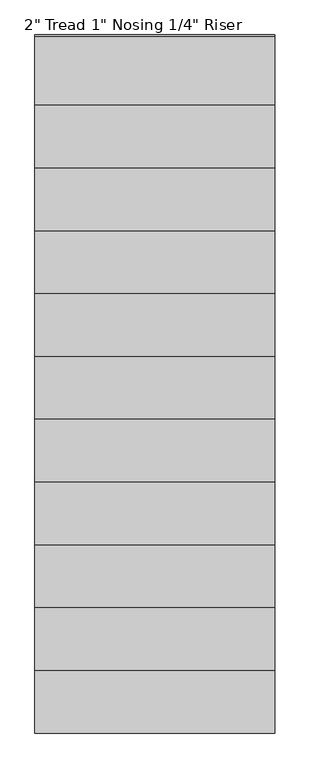
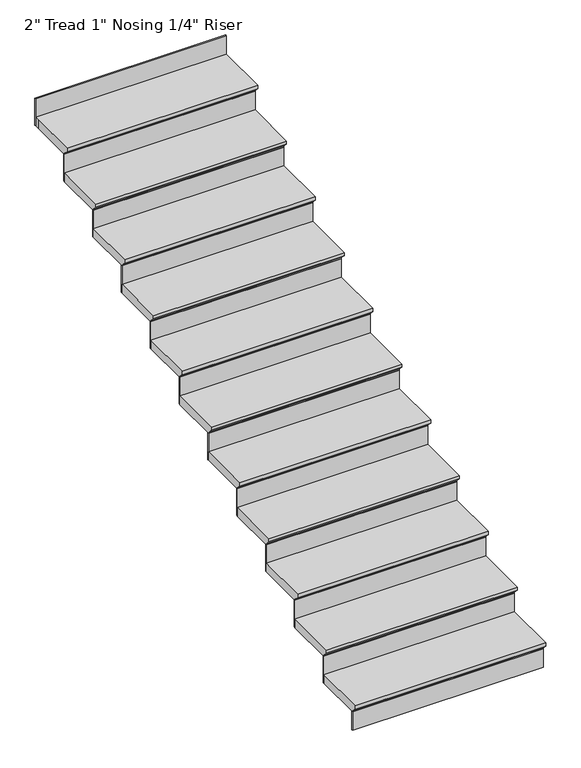
"""IFC4 building model written with IfcOpenShell, lengths in millimetres: stair flight geometry."""

from ifc_helpers import new_model, si_unit, origin, place, context, project, spatial, faceted_brep, source, transform, mapped, element, save


def stair_flight_4c38af94(model_context):
    return source(origin(), model_context, "Body", "Brep", [
        faceted_brep([(-5186.1338869, 1781.9468856, 141.3710526), (-5186.1338869, 1781.9468856, 160.4210526), (-6252.9338869, 1781.9468856, 160.4210526), (-6252.9338869, 1781.9468856, 141.3710526), (-5186.1338869, 1807.3468856, 115.9710526), (-6252.9338869, 1807.3468856, 115.9710526), (-5186.1338869, 2086.7468856, 160.4210526), (-6252.9338869, 2086.7468856, 160.4210526), (-6252.9338869, 1807.3468856, 109.6210526), (-6252.9338869, 2086.7468856, 109.6210526), (-5186.1338869, 2086.7468856, 109.6210526), (-5186.1338869, 1807.3468856, 109.6210526)], [[[0, 1, 2, 3]], [[4, 0, 3, 5]], [[2, 1, 6, 7]], [[8, 9, 10, 11]], [[2, 7, 9, 8, 5, 3]], [[8, 11, 4, 5]], [[6, 1, 0, 4, 11, 10]], [[7, 6, 10, 9]]]),
        faceted_brep([(-5186.1338869, 1807.3468856, 109.6210526), (-5186.1338869, 1807.3468856, 0.0), (-5186.1338869, 1813.6968856, 0.0), (-5186.1338869, 1813.6968856, 109.6210526), (-6252.9338869, 1807.3468856, 109.6210526), (-6252.9338869, 1813.6968856, 109.6210526), (-6252.9338869, 1813.6968856, 0.0), (-6252.9338869, 1807.3468856, 0.0)], [[[0, 1, 2, 3]], [[4, 5, 6, 7]], [[1, 0, 4, 7]], [[2, 1, 7, 6]], [[3, 2, 6, 5]], [[0, 3, 5, 4]]]),
        faceted_brep([(-5186.1338869, 2086.7468856, 270.0421053), (-5186.1338869, 2086.7468856, 109.6210526), (-5186.1338869, 2093.0968856, 109.6210526), (-5186.1338869, 2093.0968856, 270.0421053), (-6252.9338869, 2086.7468856, 270.0421053), (-6252.9338869, 2093.0968856, 270.0421053), (-6252.9338869, 2093.0968856, 109.6210526), (-6252.9338869, 2086.7468856, 109.6210526)], [[[0, 1, 2, 3]], [[4, 5, 6, 7]], [[1, 0, 4, 7]], [[2, 1, 7, 6]], [[3, 2, 6, 5]], [[0, 3, 5, 4]]]),
        faceted_brep([(-6252.9338869, 2061.3468856, 320.8421053), (-5186.1338869, 2061.3468856, 320.8421053), (-5186.1338869, 2366.1468856, 320.8421053), (-6252.9338869, 2366.1468856, 320.8421053), (-6252.9338869, 2086.7468856, 270.0421053), (-6252.9338869, 2366.1468856, 270.0421053), (-5186.1338869, 2366.1468856, 270.0421053), (-5186.1338869, 2086.7468856, 270.0421053), (-6252.9338869, 2086.7468856, 276.3921053), (-6252.9338869, 2061.3468856, 301.7921053), (-5186.1338869, 2086.7468856, 276.3921053), (-5186.1338869, 2061.3468856, 301.7921053)], [[[0, 1, 2, 3]], [[4, 5, 6, 7]], [[0, 3, 5, 4, 8, 9]], [[4, 7, 10, 8]], [[2, 1, 11, 10, 7, 6]], [[3, 2, 6, 5]], [[11, 1, 0, 9]], [[10, 11, 9, 8]]]),
        faceted_brep([(-5186.1338869, 2366.1468856, 430.4631579), (-5186.1338869, 2366.1468856, 270.0421053), (-5186.1338869, 2372.4968856, 270.0421053), (-5186.1338869, 2372.4968856, 430.4631579), (-6252.9338869, 2366.1468856, 430.4631579), (-6252.9338869, 2372.4968856, 430.4631579), (-6252.9338869, 2372.4968856, 270.0421053), (-6252.9338869, 2366.1468856, 270.0421053)], [[[0, 1, 2, 3]], [[4, 5, 6, 7]], [[1, 0, 4, 7]], [[2, 1, 7, 6]], [[3, 2, 6, 5]], [[0, 3, 5, 4]]]),
        faceted_brep([(-6252.9338869, 2340.7468856, 481.2631579), (-5186.1338869, 2340.7468856, 481.2631579), (-5186.1338869, 2645.5468856, 481.2631579), (-6252.9338869, 2645.5468856, 481.2631579), (-6252.9338869, 2366.1468856, 430.4631579), (-6252.9338869, 2645.5468856, 430.4631579), (-5186.1338869, 2645.5468856, 430.4631579), (-5186.1338869, 2366.1468856, 430.4631579), (-6252.9338869, 2366.1468856, 436.8131579), (-6252.9338869, 2340.7468856, 462.2131579), (-5186.1338869, 2366.1468856, 436.8131579), (-5186.1338869, 2340.7468856, 462.2131579)], [[[0, 1, 2, 3]], [[4, 5, 6, 7]], [[0, 3, 5, 4, 8, 9]], [[4, 7, 10, 8]], [[2, 1, 11, 10, 7, 6]], [[3, 2, 6, 5]], [[11, 1, 0, 9]], [[10, 11, 9, 8]]]),
        faceted_brep([(-5186.1338869, 2645.5468856, 590.8842105), (-5186.1338869, 2645.5468856, 430.4631579), (-5186.1338869, 2651.8968856, 430.4631579), (-5186.1338869, 2651.8968856, 590.8842105), (-6252.9338869, 2645.5468856, 590.8842105), (-6252.9338869, 2651.8968856, 590.8842105), (-6252.9338869, 2651.8968856, 430.4631579), (-6252.9338869, 2645.5468856, 430.4631579)], [[[0, 1, 2, 3]], [[4, 5, 6, 7]], [[1, 0, 4, 7]], [[2, 1, 7, 6]], [[3, 2, 6, 5]], [[0, 3, 5, 4]]]),
        faceted_brep([(-6252.9338869, 2620.1468856, 641.6842105), (-5186.1338869, 2620.1468856, 641.6842105), (-5186.1338869, 2924.9468856, 641.6842105), (-6252.9338869, 2924.9468856, 641.6842105), (-6252.9338869, 2645.5468856, 590.8842105), (-6252.9338869, 2924.9468856, 590.8842105), (-5186.1338869, 2924.9468856, 590.8842105), (-5186.1338869, 2645.5468856, 590.8842105), (-6252.9338869, 2645.5468856, 597.2342105), (-6252.9338869, 2620.1468856, 622.6342105), (-5186.1338869, 2645.5468856, 597.2342105), (-5186.1338869, 2620.1468856, 622.6342105)], [[[0, 1, 2, 3]], [[4, 5, 6, 7]], [[0, 3, 5, 4, 8, 9]], [[4, 7, 10, 8]], [[2, 1, 11, 10, 7, 6]], [[3, 2, 6, 5]], [[11, 1, 0, 9]], [[10, 11, 9, 8]]]),
        faceted_brep([(-5186.1338869, 2924.9468856, 751.3052632), (-5186.1338869, 2924.9468856, 590.8842105), (-5186.1338869, 2931.2968856, 590.8842105), (-5186.1338869, 2931.2968856, 751.3052632), (-6252.9338869, 2924.9468856, 751.3052632), (-6252.9338869, 2931.2968856, 751.3052632), (-6252.9338869, 2931.2968856, 590.8842105), (-6252.9338869, 2924.9468856, 590.8842105)], [[[0, 1, 2, 3]], [[4, 5, 6, 7]], [[1, 0, 4, 7]], [[2, 1, 7, 6]], [[3, 2, 6, 5]], [[0, 3, 5, 4]]]),
        faceted_brep([(-6252.9338869, 2899.5468856, 802.1052632), (-5186.1338869, 2899.5468856, 802.1052632), (-5186.1338869, 3204.3468856, 802.1052632), (-6252.9338869, 3204.3468856, 802.1052632), (-6252.9338869, 2924.9468856, 751.3052632), (-6252.9338869, 3204.3468856, 751.3052632), (-5186.1338869, 3204.3468856, 751.3052632), (-5186.1338869, 2924.9468856, 751.3052632), (-6252.9338869, 2924.9468856, 757.6552632), (-6252.9338869, 2899.5468856, 783.0552632), (-5186.1338869, 2924.9468856, 757.6552632), (-5186.1338869, 2899.5468856, 783.0552632)], [[[0, 1, 2, 3]], [[4, 5, 6, 7]], [[0, 3, 5, 4, 8, 9]], [[4, 7, 10, 8]], [[2, 1, 11, 10, 7, 6]], [[3, 2, 6, 5]], [[11, 1, 0, 9]], [[10, 11, 9, 8]]]),
        faceted_brep([(-5186.1338869, 3204.3468856, 911.7263158), (-5186.1338869, 3204.3468856, 751.3052632), (-5186.1338869, 3210.6968856, 751.3052632), (-5186.1338869, 3210.6968856, 911.7263158), (-6252.9338869, 3204.3468856, 911.7263158), (-6252.9338869, 3210.6968856, 911.7263158), (-6252.9338869, 3210.6968856, 751.3052632), (-6252.9338869, 3204.3468856, 751.3052632)], [[[0, 1, 2, 3]], [[4, 5, 6, 7]], [[1, 0, 4, 7]], [[2, 1, 7, 6]], [[3, 2, 6, 5]], [[0, 3, 5, 4]]]),
        faceted_brep([(-6252.9338869, 3178.9468856, 962.5263158), (-5186.1338869, 3178.9468856, 962.5263158), (-5186.1338869, 3483.7468856, 962.5263158), (-6252.9338869, 3483.7468856, 962.5263158), (-6252.9338869, 3204.3468856, 911.7263158), (-6252.9338869, 3483.7468856, 911.7263158), (-5186.1338869, 3483.7468856, 911.7263158), (-5186.1338869, 3204.3468856, 911.7263158), (-6252.9338869, 3204.3468856, 918.0763158), (-6252.9338869, 3178.9468856, 943.4763158), (-5186.1338869, 3204.3468856, 918.0763158), (-5186.1338869, 3178.9468856, 943.4763158)], [[[0, 1, 2, 3]], [[4, 5, 6, 7]], [[0, 3, 5, 4, 8, 9]], [[4, 7, 10, 8]], [[2, 1, 11, 10, 7, 6]], [[3, 2, 6, 5]], [[11, 1, 0, 9]], [[10, 11, 9, 8]]]),
        faceted_brep([(-5186.1338869, 3483.7468856, 1072.1473684), (-5186.1338869, 3483.7468856, 911.7263158), (-5186.1338869, 3490.0968856, 911.7263158), (-5186.1338869, 3490.0968856, 1072.1473684), (-6252.9338869, 3483.7468856, 1072.1473684), (-6252.9338869, 3490.0968856, 1072.1473684), (-6252.9338869, 3490.0968856, 911.7263158), (-6252.9338869, 3483.7468856, 911.7263158)], [[[0, 1, 2, 3]], [[4, 5, 6, 7]], [[1, 0, 4, 7]], [[2, 1, 7, 6]], [[3, 2, 6, 5]], [[0, 3, 5, 4]]]),
        faceted_brep([(-6252.9338869, 3458.3468856, 1122.9473684), (-5186.1338869, 3458.3468856, 1122.9473684), (-5186.1338869, 3763.1468856, 1122.9473684), (-6252.9338869, 3763.1468856, 1122.9473684), (-6252.9338869, 3483.7468856, 1072.1473684), (-6252.9338869, 3763.1468856, 1072.1473684), (-5186.1338869, 3763.1468856, 1072.1473684), (-5186.1338869, 3483.7468856, 1072.1473684), (-6252.9338869, 3483.7468856, 1078.4973684), (-6252.9338869, 3458.3468856, 1103.8973684), (-5186.1338869, 3483.7468856, 1078.4973684), (-5186.1338869, 3458.3468856, 1103.8973684)], [[[0, 1, 2, 3]], [[4, 5, 6, 7]], [[0, 3, 5, 4, 8, 9]], [[4, 7, 10, 8]], [[2, 1, 11, 10, 7, 6]], [[3, 2, 6, 5]], [[11, 1, 0, 9]], [[10, 11, 9, 8]]]),
        faceted_brep([(-5186.1338869, 3763.1468856, 1232.5684211), (-5186.1338869, 3763.1468856, 1072.1473684), (-5186.1338869, 3769.4968856, 1072.1473684), (-5186.1338869, 3769.4968856, 1232.5684211), (-6252.9338869, 3763.1468856, 1232.5684211), (-6252.9338869, 3769.4968856, 1232.5684211), (-6252.9338869, 3769.4968856, 1072.1473684), (-6252.9338869, 3763.1468856, 1072.1473684)], [[[0, 1, 2, 3]], [[4, 5, 6, 7]], [[1, 0, 4, 7]], [[2, 1, 7, 6]], [[3, 2, 6, 5]], [[0, 3, 5, 4]]]),
        faceted_brep([(-6252.9338869, 3737.7468856, 1283.3684211), (-5186.1338869, 3737.7468856, 1283.3684211), (-5186.1338869, 4042.5468856, 1283.3684211), (-6252.9338869, 4042.5468856, 1283.3684211), (-6252.9338869, 3763.1468856, 1232.5684211), (-6252.9338869, 4042.5468856, 1232.5684211), (-5186.1338869, 4042.5468856, 1232.5684211), (-5186.1338869, 3763.1468856, 1232.5684211), (-6252.9338869, 3763.1468856, 1238.9184211), (-6252.9338869, 3737.7468856, 1264.3184211), (-5186.1338869, 3763.1468856, 1238.9184211), (-5186.1338869, 3737.7468856, 1264.3184211)], [[[0, 1, 2, 3]], [[4, 5, 6, 7]], [[0, 3, 5, 4, 8, 9]], [[4, 7, 10, 8]], [[2, 1, 11, 10, 7, 6]], [[3, 2, 6, 5]], [[11, 1, 0, 9]], [[10, 11, 9, 8]]]),
        faceted_brep([(-5186.1338869, 4042.5468856, 1392.9894737), (-5186.1338869, 4042.5468856, 1232.5684211), (-5186.1338869, 4048.8968856, 1232.5684211), (-5186.1338869, 4048.8968856, 1392.9894737), (-6252.9338869, 4042.5468856, 1392.9894737), (-6252.9338869, 4048.8968856, 1392.9894737), (-6252.9338869, 4048.8968856, 1232.5684211), (-6252.9338869, 4042.5468856, 1232.5684211)], [[[0, 1, 2, 3]], [[4, 5, 6, 7]], [[1, 0, 4, 7]], [[2, 1, 7, 6]], [[3, 2, 6, 5]], [[0, 3, 5, 4]]]),
        faceted_brep([(-6252.9338869, 4017.1468856, 1443.7894737), (-5186.1338869, 4017.1468856, 1443.7894737), (-5186.1338869, 4321.9468856, 1443.7894737), (-6252.9338869, 4321.9468856, 1443.7894737), (-6252.9338869, 4042.5468856, 1392.9894737), (-6252.9338869, 4321.9468856, 1392.9894737), (-5186.1338869, 4321.9468856, 1392.9894737), (-5186.1338869, 4042.5468856, 1392.9894737), (-6252.9338869, 4042.5468856, 1399.3394737), (-6252.9338869, 4017.1468856, 1424.7394737), (-5186.1338869, 4042.5468856, 1399.3394737), (-5186.1338869, 4017.1468856, 1424.7394737)], [[[0, 1, 2, 3]], [[4, 5, 6, 7]], [[0, 3, 5, 4, 8, 9]], [[4, 7, 10, 8]], [[2, 1, 11, 10, 7, 6]], [[3, 2, 6, 5]], [[11, 1, 0, 9]], [[10, 11, 9, 8]]]),
        faceted_brep([(-5186.1338869, 4321.9468856, 1553.4105263), (-5186.1338869, 4321.9468856, 1392.9894737), (-5186.1338869, 4328.2968856, 1392.9894737), (-5186.1338869, 4328.2968856, 1553.4105263), (-6252.9338869, 4321.9468856, 1553.4105263), (-6252.9338869, 4328.2968856, 1553.4105263), (-6252.9338869, 4328.2968856, 1392.9894737), (-6252.9338869, 4321.9468856, 1392.9894737)], [[[0, 1, 2, 3]], [[4, 5, 6, 7]], [[1, 0, 4, 7]], [[2, 1, 7, 6]], [[3, 2, 6, 5]], [[0, 3, 5, 4]]]),
        faceted_brep([(-6252.9338869, 4296.5468856, 1604.2105263), (-5186.1338869, 4296.5468856, 1604.2105263), (-5186.1338869, 4601.3468856, 1604.2105263), (-6252.9338869, 4601.3468856, 1604.2105263), (-6252.9338869, 4321.9468856, 1553.4105263), (-6252.9338869, 4601.3468856, 1553.4105263), (-5186.1338869, 4601.3468856, 1553.4105263), (-5186.1338869, 4321.9468856, 1553.4105263), (-6252.9338869, 4321.9468856, 1559.7605263), (-6252.9338869, 4296.5468856, 1585.1605263), (-5186.1338869, 4321.9468856, 1559.7605263), (-5186.1338869, 4296.5468856, 1585.1605263)], [[[0, 1, 2, 3]], [[4, 5, 6, 7]], [[0, 3, 5, 4, 8, 9]], [[4, 7, 10, 8]], [[2, 1, 11, 10, 7, 6]], [[3, 2, 6, 5]], [[11, 1, 0, 9]], [[10, 11, 9, 8]]]),
        faceted_brep([(-5186.1338869, 4880.7468856, 1874.2526316), (-5186.1338869, 4880.7468856, 1713.8315789), (-5186.1338869, 4887.0968856, 1713.8315789), (-5186.1338869, 4887.0968856, 1874.2526316), (-6252.9338869, 4880.7468856, 1874.2526316), (-6252.9338869, 4887.0968856, 1874.2526316), (-6252.9338869, 4887.0968856, 1713.8315789), (-6252.9338869, 4880.7468856, 1713.8315789)], [[[0, 1, 2, 3]], [[4, 5, 6, 7]], [[1, 0, 4, 7]], [[2, 1, 7, 6]], [[3, 2, 6, 5]], [[0, 3, 5, 4]]]),
        faceted_brep([(-5186.1338869, 4601.3468856, 1713.8315789), (-5186.1338869, 4601.3468856, 1553.4105263), (-5186.1338869, 4607.6968856, 1553.4105263), (-5186.1338869, 4607.6968856, 1713.8315789), (-6252.9338869, 4601.3468856, 1713.8315789), (-6252.9338869, 4607.6968856, 1713.8315789), (-6252.9338869, 4607.6968856, 1553.4105263), (-6252.9338869, 4601.3468856, 1553.4105263)], [[[0, 1, 2, 3]], [[4, 5, 6, 7]], [[1, 0, 4, 7]], [[2, 1, 7, 6]], [[3, 2, 6, 5]], [[0, 3, 5, 4]]]),
        faceted_brep([(-6252.9338869, 4880.7468856, 1764.6315789), (-6252.9338869, 4855.3468856, 1764.6315789), (-6252.9338869, 4575.9468856, 1764.6315789), (-5186.1338869, 4575.9468856, 1764.6315789), (-5186.1338869, 4880.7468856, 1764.6315789), (-6252.9338869, 4855.3468856, 1713.8315789), (-6252.9338869, 4880.7468856, 1713.8315789), (-5186.1338869, 4880.7468856, 1713.8315789), (-5186.1338869, 4601.3468856, 1713.8315789), (-6252.9338869, 4601.3468856, 1713.8315789), (-6252.9338869, 4601.3468856, 1720.1815789), (-6252.9338869, 4575.9468856, 1745.5815789), (-5186.1338869, 4601.3468856, 1720.1815789), (-5186.1338869, 4575.9468856, 1745.5815789)], [[[0, 1, 2, 3, 4]], [[5, 6, 7, 8, 9]], [[1, 0, 6, 5]], [[2, 1, 5, 9, 10, 11]], [[9, 8, 12, 10]], [[4, 3, 13, 12, 8, 7]], [[0, 4, 7, 6]], [[13, 3, 2, 11]], [[12, 13, 11, 10]]]),
    ])


if __name__ == "__main__":
    model = new_model("IFC4")
    model_context = context("Model", 3, world=origin())
    ifc_project = project(units=[si_unit("LENGTHUNIT", "METRE", prefix="MILLI")], contexts=[model_context])
    site = spatial("IfcSite", under=ifc_project)
    building = spatial("IfcBuilding", under=site)
    placement = place(None, origin())
    stair_flight_shape = stair_flight_4c38af94(model_context)
    element("IfcStairFlight", 1, ObjectType="2\" Tread 1\" Nosing 1/4\" Riser", at=placement, inside=building, context=model_context, shape_type="MappedRepresentation", body=[
        mapped(stair_flight_shape, transform((0.0, 0.0, 0.0), x_axis=(1.0, 0.0, 0.0), y_axis=(0.0, 1.0, 0.0), z_axis=(0.0, 0.0, 1.0))),
    ])
    save(model, "model.ifc")
